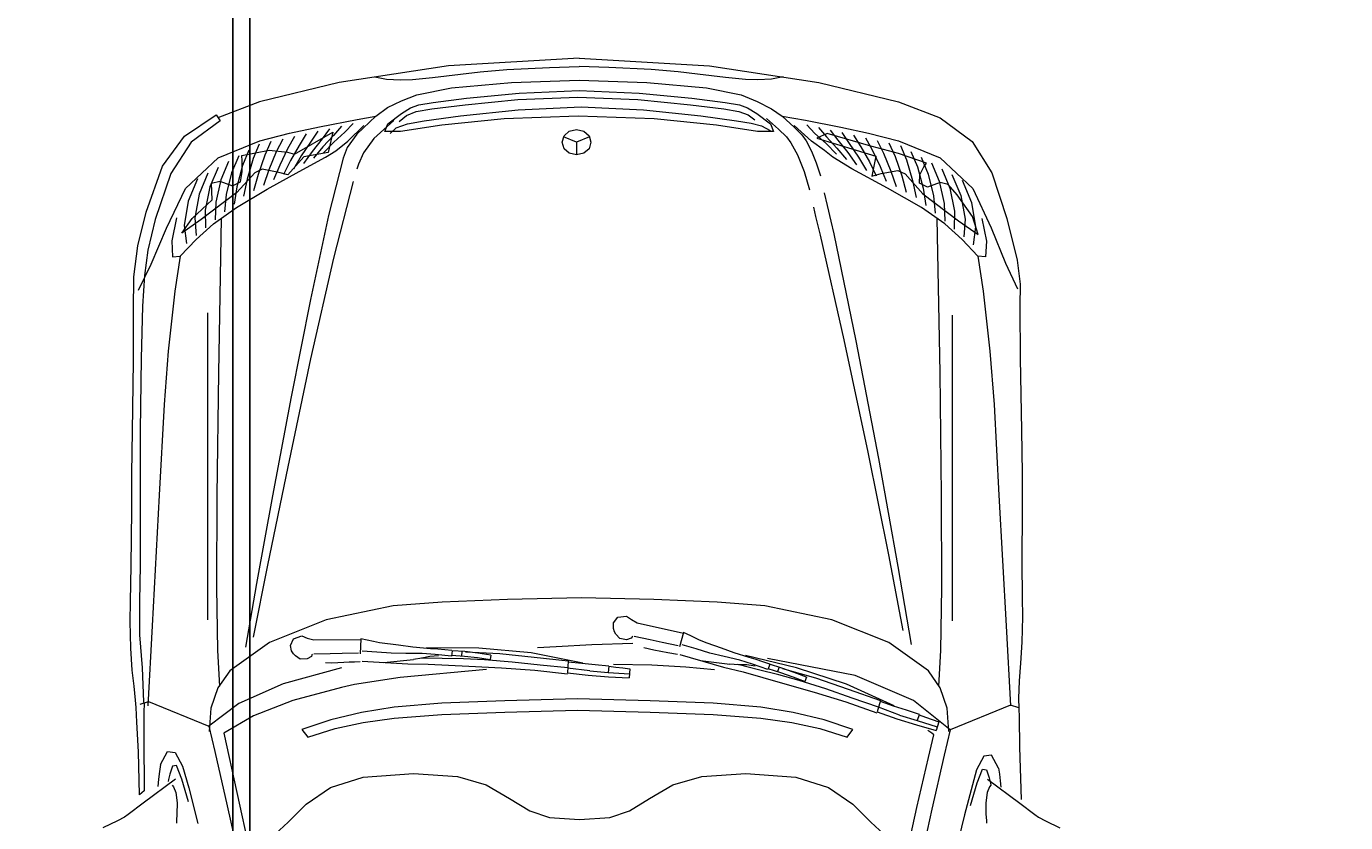
# Model space of a CAD drawing. Units: inches. Extents: x -10 to 502, y -868 to 56.
# Tile 5 of 14: x 78 to 165, y -626 to -573. Entities that reach past the tile are written whole.
import ezdxf

# ---------------------------------------------------------------- set-up
doc = ezdxf.new("R2010")
doc.units = ezdxf.units.IN
doc.header["$MEASUREMENT"] = 0
doc.layers.add('A-ANNO-DIMS', color=2, linetype='Continuous', lineweight=18)
doc.layers.add('C-PRKG-VEHI', color=8, linetype='Continuous', lineweight=13)
doc.styles.get("Standard").update_dxf_attribs({"font": 'arial.ttf'})
doc.dimstyles.get("Standard").update_dxf_attribs({"dimtxt": 0.18, "dimasz": 0.18, "dimexe": 0.18, "dimexo": 0.0625, "dimgap": 0.09, "dimtad": 0, "dimtih": 1, "dimtoh": 1, "dimdec": 0, "dimzin": 0, "dimdsep": 46, "dimlunit": 3, "dimtxsty": 'Standard', "dimcen": 0.09, "dimadec": 0, "dimazin": 0, "dimtfac": 1, "dimtdec": 0, "dimtofl": 0, "dimtmove": 0, "dimatfit": 3, "dimfxl": 1, "dimtolj": 1, "dimtzin": 0, "dimarcsym": 0})

# ---------------------------------------------------------------- blocks, each defined once
blk = doc.blocks.new('*D47')
at = {"layer": 'A-ANNO-DIMS', "color": 0, "lineweight": -2, "transparency": 16777216}
for p, q in [((91.951, -494.915), (91.951, -846.583)), ((201.951, -494.915), (201.951, -846.583)), ((92.131, -846.403), (146.622, -846.403)), ((201.771, -846.403), (147.28, -846.403))]:
    blk.add_line(p, q, dxfattribs=at)
at = {"layer": 'A-ANNO-DIMS', "color": 0, "transparency": 16777216}
for points in [[(92.131, -846.373), (92.131, -846.433), (91.951, -846.403)], [(201.771, -846.373), (201.771, -846.433), (201.951, -846.403)]]:
    blk.add_solid(points, dxfattribs=at)
at = {"layer": 'Defpoints', "color": 0, "transparency": 16777216}
for p in [(91.951, -494.853), (201.951, -494.853), (201.951, -846.403)]:
    blk.add_point(p, dxfattribs=at)
at = {"layer": 'A-ANNO-DIMS', "color": 0, "transparency": 16777216, "insert": (146.951, -846.403), "char_height": 0.18, "attachment_point": 5}
blk.add_mtext('\\A1;9\'-2"', dxfattribs=at)
blk = doc.blocks.new('*D56')
at = {"layer": 'A-ANNO-DIMS', "color": 0, "lineweight": -2, "transparency": 16777216}
for p, q in [((43.951, -549.915), (43.951, -846.583)), ((93.073, -549.915), (93.073, -846.583)), ((44.131, -846.403), (68.179, -846.403)), ((92.893, -846.403), (68.845, -846.403))]:
    blk.add_line(p, q, dxfattribs=at)
at = {"layer": 'A-ANNO-DIMS', "color": 0, "transparency": 16777216}
for points in [[(44.131, -846.373), (44.131, -846.433), (43.951, -846.403)], [(92.893, -846.373), (92.893, -846.433), (93.073, -846.403)]]:
    blk.add_solid(points, dxfattribs=at)
at = {"layer": 'Defpoints', "color": 0, "transparency": 16777216}
for p in [(43.951, -549.853), (93.073, -549.853), (43.951, -846.403)]:
    blk.add_point(p, dxfattribs=at)
at = {"layer": 'A-ANNO-DIMS', "color": 0, "transparency": 16777216, "insert": (68.512, -846.403), "char_height": 0.18, "attachment_point": 5}
blk.add_mtext('\\A1;4\'-1"', dxfattribs=at)

msp = doc.modelspace()

# ---------------------------------------------------------------- linework, layer by layer
at = {"layer": 'C-PRKG-VEHI'}
for p, q in [((106.171, -576.058), (98.969, -577.156)), ((114.77, -575.546), (106.171, -576.058)), ((110.011, -576.309), (112.816, -576.171)), ((112.816, -576.171), (114.77, -576.109)), ((114.77, -575.546), (123.37, -576.058)), ((116.725, -576.171), (114.77, -576.109)), ((119.529, -576.309), (116.725, -576.171)), ((123.37, -576.058), (130.572, -577.156)), ((101.325, -576.784), (102.091, -576.94)), ((102.091, -576.94), (102.996, -576.984)), ((102.996, -576.984), (103.8, -576.952)), ((103.8, -576.952), (105.115, -576.821)), ((105.115, -576.821), (106.967, -576.615)), ((106.967, -576.615), (108.245, -576.446)), ((108.245, -576.446), (110.011, -576.309)), ((110.311, -577.157), (114.77, -577.009)), ((114.77, -577.009), (119.229, -577.157)), ((121.296, -576.446), (119.529, -576.309)), ((122.574, -576.615), (121.296, -576.446)), ((124.426, -576.821), (122.574, -576.615)), ((125.74, -576.952), (124.426, -576.821)), ((126.545, -576.984), (125.74, -576.952)), ((127.449, -576.94), (126.545, -576.984)), ((128.216, -576.784), (127.449, -576.94)), ((98.969, -577.156), (93.718, -578.434)), ((104.081, -577.965), (106.365, -577.517)), ((106.365, -577.517), (110.311, -577.157)), ((107.344, -578.192), (110.814, -577.851)), ((110.814, -577.851), (114.77, -577.684)), ((114.77, -577.684), (118.727, -577.851)), ((118.727, -577.851), (122.196, -578.192)), ((119.229, -577.157), (123.176, -577.517)), ((123.176, -577.517), (125.459, -577.965)), ((130.572, -577.156), (135.822, -578.434)), ((93.718, -578.434), (90.973, -579.484)), ((102.159, -578.803), (103.064, -578.378)), ((103.064, -578.378), (104.081, -577.965)), ((103.665, -578.833), (104.208, -578.627)), ((104.208, -578.627), (105.15, -578.471)), ((105.064, -578.905), (107.258, -578.626)), ((105.15, -578.471), (107.344, -578.192)), ((107.258, -578.626), (110.727, -578.284)), ((110.727, -578.284), (114.684, -578.117)), ((110.76, -578.965), (114.9, -578.767)), ((114.684, -578.117), (118.641, -578.284)), ((114.9, -578.767), (119.02, -578.965)), ((118.641, -578.284), (122.11, -578.626)), ((122.11, -578.626), (124.304, -578.905)), ((122.196, -578.192), (124.391, -578.471)), ((124.391, -578.471), (125.333, -578.627)), ((125.333, -578.627), (125.876, -578.833)), ((125.459, -577.965), (126.507, -578.421)), ((126.507, -578.421), (127.442, -578.89)), ((135.822, -578.434), (138.568, -579.484)), ((88.776, -580.703), (90.853, -579.285)), ((90.853, -579.285), (91.128, -579.68)), ((97.672, -580.08), (100.158, -579.601)), ((101.381, -579.372), (100.134, -580.564)), ((100.158, -579.601), (101.381, -579.372)), ((102.557, -579.662), (101.252, -580.855)), ((101.381, -579.372), (102.159, -578.803)), ((102.166, -579.884), (103.069, -579.203)), ((102.925, -579.74), (103.394, -579.33)), ((103.069, -579.203), (103.665, -578.833)), ((103.394, -579.33), (104.035, -579.081)), ((104.035, -579.081), (105.064, -578.905)), ((104.571, -579.675), (106.949, -579.365)), ((109.825, -579.559), (105.737, -579.972)), ((106.949, -579.365), (110.76, -578.965)), ((114.714, -579.372), (109.825, -579.559)), ((119.727, -579.559), (114.714, -579.372)), ((119.02, -578.965), (122.792, -579.365)), ((123.822, -579.972), (119.727, -579.559)), ((122.792, -579.365), (125.149, -579.675)), ((124.304, -578.905), (125.301, -579.075)), ((125.301, -579.075), (125.903, -579.291)), ((125.876, -578.833), (126.472, -579.203)), ((125.903, -579.291), (126.345, -579.61)), ((126.472, -579.203), (127.374, -579.884)), ((127.12, -579.525), (127.903, -580.235)), ((127.442, -578.89), (128.16, -579.372)), ((128.16, -579.372), (128.931, -580.095)), ((128.16, -579.372), (129.695, -579.644)), ((129.695, -579.644), (132.025, -580.102)), ((138.568, -579.484), (140.669, -581.054)), ((91.128, -579.68), (89.215, -581.09)), ((93.732, -580.995), (95.699, -580.497)), ((95.699, -580.497), (97.672, -580.08)), ((96.025, -581.894), (98.543, -580.432)), ((97.567, -580.376), (97.083, -581.086)), ((98.34, -580.205), (97.838, -580.869)), ((98.543, -580.432), (98.235, -581.764)), ((99.114, -580.035), (98.593, -580.651)), ((99.348, -580.434), (98.605, -581.086)), ((99.887, -579.864), (99.348, -580.434)), ((99.536, -581.022), (100.593, -579.991)), ((101.964, -580.378), (102.166, -579.884)), ((103.012, -580.384), (101.964, -580.378)), ((102.319, -580.517), (102.711, -580.155)), ((102.711, -580.155), (103.46, -579.878)), ((105.737, -579.972), (103.012, -580.384)), ((103.46, -579.878), (104.571, -579.675)), ((113.787, -580.677), (114.127, -580.377)), ((114.127, -580.377), (114.607, -580.263)), ((114.607, -580.263), (115.086, -580.377)), ((115.086, -580.377), (115.427, -580.677)), ((126.528, -580.384), (123.822, -579.972)), ((125.149, -579.675), (126.11, -579.829)), ((126.11, -579.829), (126.787, -580.026)), ((127.576, -580.378), (126.528, -580.384)), ((126.787, -580.026), (127.358, -580.325)), ((127.374, -579.884), (127.576, -580.378)), ((127.903, -580.235), (128.433, -580.748)), ((128.931, -580.095), (129.452, -580.618)), ((130.079, -581.018), (128.948, -579.991)), ((129.767, -579.951), (130.306, -580.521)), ((130.306, -580.521), (131.049, -581.173)), ((131.111, -580.519), (130.424, -580.823)), ((130.54, -580.121), (131.061, -580.738)), ((133.985, -581.357), (131.111, -580.519)), ((131.313, -580.292), (131.816, -580.955)), ((132.025, -580.102), (133.842, -580.497)), ((132.086, -580.462), (132.571, -581.173)), ((133.842, -580.497), (135.809, -580.995)), ((87.339, -582.685), (88.776, -580.703)), ((89.215, -581.09), (87.884, -583.153)), ((90.99, -582.118), (93.732, -580.995)), ((93.702, -581.228), (93.307, -582.173)), ((94.474, -581.058), (94.062, -581.955)), ((95.248, -580.887), (94.817, -581.738)), ((96.021, -580.717), (95.572, -581.521)), ((96.327, -581.303), (95.76, -582.309)), ((96.794, -580.546), (96.327, -581.303)), ((97.083, -581.086), (96.471, -582.003)), ((97.838, -580.869), (97.182, -581.697)), ((97.894, -581.392), (97.272, -582.151)), ((98.593, -580.651), (97.894, -581.392)), ((98.605, -581.086), (97.928, -581.794)), ((98.741, -581.654), (99.536, -581.022)), ((100.134, -580.564), (99.503, -581.439)), ((101.252, -580.855), (100.559, -581.792)), ((113.657, -581.1), (113.787, -580.677)), ((113.787, -581.522), (113.657, -581.1)), ((114.607, -581.1), (113.755, -580.737)), ((115.458, -580.737), (114.607, -581.1)), ((114.607, -581.1), (114.607, -581.937)), ((115.427, -580.677), (115.556, -581.1)), ((115.556, -581.1), (115.427, -581.522)), ((128.433, -580.748), (128.723, -581.129)), ((128.723, -581.129), (129.157, -581.935)), ((129.452, -580.618), (129.735, -581.003)), ((129.735, -581.003), (130.093, -581.679)), ((130.948, -581.645), (130.079, -581.018)), ((130.424, -580.823), (134.315, -582.018)), ((131.049, -581.173), (131.725, -581.88)), ((131.061, -580.738), (131.76, -581.478)), ((131.816, -580.955), (132.471, -581.784)), ((132.571, -581.173), (133.182, -582.09)), ((132.859, -580.633), (133.326, -581.39)), ((133.326, -581.39), (133.893, -582.396)), ((133.632, -580.803), (134.081, -581.607)), ((134.488, -581.478), (133.985, -581.357)), ((134.405, -580.974), (134.836, -581.825)), ((135.179, -581.144), (135.591, -582.042)), ((135.809, -580.995), (138.551, -582.118)), ((135.952, -581.315), (136.346, -582.259)), ((140.669, -581.054), (141.962, -583.107)), ((88.835, -584.154), (90.99, -582.118)), ((92.348, -581.992), (91.881, -583.11)), ((92.56, -581.98), (94.351, -581.619)), ((92.583, -582.325), (92.56, -581.98)), ((93.025, -581.61), (92.594, -582.641)), ((93.307, -582.173), (92.915, -583.532)), ((94.062, -581.955), (93.626, -583.226)), ((94.817, -581.738), (94.338, -582.92)), ((94.351, -581.619), (95.573, -581.747)), ((95.572, -581.521), (95.049, -582.615)), ((95.573, -581.747), (96.025, -581.894)), ((96.632, -582.067), (95.592, -583.255)), ((96.471, -582.003), (95.958, -582.866)), ((96.341, -583.018), (98.062, -582.072)), ((97.182, -581.697), (96.615, -582.509)), ((98.235, -581.764), (96.632, -582.067)), ((98.062, -582.072), (98.741, -581.654)), ((99.225, -582.146), (98.272, -585.933)), ((99.503, -581.439), (99.225, -582.146)), ((100.559, -581.792), (100.239, -582.534)), ((114.127, -581.823), (113.787, -581.522)), ((114.607, -581.937), (114.127, -581.823)), ((115.086, -581.823), (114.607, -581.937)), ((115.427, -581.522), (115.086, -581.823)), ((129.157, -581.935), (129.6, -583.019)), ((130.093, -581.679), (130.4, -582.452)), ((131.479, -582.072), (130.948, -581.645)), ((132.746, -582.858), (131.479, -582.072)), ((131.76, -581.478), (132.382, -582.238)), ((132.471, -581.784), (133.038, -582.595)), ((133.182, -582.09), (133.695, -582.953)), ((134.315, -582.018), (134.061, -583.342)), ((134.081, -581.607), (134.604, -582.701)), ((135.805, -581.847), (134.488, -581.478)), ((134.836, -581.825), (135.316, -583.007)), ((135.591, -582.042), (136.027, -583.313)), ((137.647, -582.476), (135.805, -581.847)), ((136.346, -582.259), (136.738, -583.619)), ((136.629, -581.697), (137.059, -582.728)), ((137.306, -582.078), (137.772, -583.197)), ((138.551, -582.118), (140.705, -584.154)), ((86.246, -585.697), (87.339, -582.685)), ((90.317, -583.137), (89.742, -584.516)), ((90.994, -582.756), (90.455, -584.047)), ((91.671, -582.374), (91.168, -583.579)), ((91.881, -583.11), (91.531, -584.548)), ((92.594, -582.641), (92.223, -584.04)), ((93.404, -583.103), (92.235, -584.407)), ((92.464, -583.717), (92.585, -583.055)), ((92.585, -583.055), (92.583, -582.325)), ((93.894, -582.873), (93.404, -583.103)), ((94.986, -583.081), (93.894, -582.873)), ((94.338, -582.92), (93.988, -583.939)), ((94.226, -584.198), (96.341, -583.018)), ((95.049, -582.615), (94.645, -583.581)), ((95.592, -583.255), (94.986, -583.081)), ((95.76, -582.309), (95.301, -583.224)), ((100.239, -582.534), (100.126, -582.88)), ((129.6, -583.019), (129.957, -584.224)), ((130.4, -582.452), (130.668, -583.303)), ((135.088, -584.118), (132.746, -582.858)), ((133.893, -582.396), (134.352, -583.31)), ((134.604, -582.701), (135.009, -583.668)), ((134.667, -583.168), (135.759, -582.959)), ((135.316, -583.007), (135.665, -584.025)), ((135.759, -582.959), (136.249, -583.189)), ((137.059, -582.728), (137.431, -584.127)), ((137.212, -583.248), (137.48, -582.714)), ((137.48, -582.714), (137.647, -582.476)), ((137.983, -582.46), (138.485, -583.665)), ((138.659, -582.842), (139.198, -584.134)), ((141.962, -583.107), (142.956, -586.123)), ((87.884, -583.153), (86.835, -586.192)), ((89.64, -583.519), (89.029, -584.984)), ((90.561, -583.793), (91.1, -583.656)), ((90.603, -584.893), (90.561, -583.793)), ((91.168, -583.579), (90.838, -585.057)), ((91.1, -583.656), (91.936, -583.981)), ((91.936, -583.981), (92.464, -583.717)), ((92.915, -583.532), (92.674, -584.654)), ((93.626, -583.226), (93.331, -584.296)), ((99.883, -583.683), (98.586, -588.74)), ((134.061, -583.342), (134.667, -583.168)), ((136.027, -583.313), (136.322, -584.383)), ((136.249, -583.189), (137.419, -584.494)), ((136.738, -583.619), (136.979, -584.74)), ((137.19, -583.804), (137.212, -583.248)), ((137.718, -584.068), (137.19, -583.804)), ((138.553, -583.742), (137.718, -584.068)), ((137.772, -583.197), (138.123, -584.635)), ((138.485, -583.665), (138.815, -585.143)), ((139.092, -583.88), (138.553, -583.742)), ((139.669, -584.573), (139.092, -583.88)), ((139.336, -583.224), (139.911, -584.602)), ((140.014, -583.606), (140.624, -585.071)), ((87.583, -586.764), (88.835, -584.154)), ((89.742, -584.516), (89.453, -586.073)), ((92.235, -584.407), (89.881, -586.195)), ((90.455, -584.047), (90.146, -585.565)), ((91.531, -584.548), (91.42, -585.694)), ((92.223, -584.04), (92.047, -585.174)), ((92.211, -585.391), (94.226, -584.198)), ((130.91, -584.441), (131.105, -585.276)), ((137.33, -585.391), (135.088, -584.118)), ((137.419, -584.494), (139.772, -586.282)), ((137.431, -584.127), (137.606, -585.26)), ((138.123, -584.635), (138.233, -585.78)), ((139.198, -584.134), (139.508, -585.651)), ((140.682, -585.999), (139.669, -584.573)), ((139.911, -584.602), (140.2, -586.16)), ((140.705, -584.154), (141.92, -586.739)), ((85.712, -587.928), (86.246, -585.697)), ((89.029, -584.984), (88.761, -586.581)), ((89.28, -586.116), (90.603, -584.893)), ((90.146, -585.565), (90.167, -586.735)), ((90.686, -586.473), (92.211, -585.391)), ((90.838, -585.057), (90.794, -586.214)), ((130.209, -585.367), (130.354, -585.986)), ((131.105, -585.276), (131.352, -586.299)), ((138.855, -586.473), (137.33, -585.391)), ((138.815, -585.143), (138.86, -586.301)), ((139.508, -585.651), (139.487, -586.821)), ((140.624, -585.071), (140.892, -586.668)), ((86.835, -586.192), (86.356, -588.21)), ((88.249, -586.08), (87.944, -587.593)), ((88.596, -587.095), (89.28, -586.116)), ((89.881, -586.195), (88.596, -587.095)), ((88.761, -586.581), (88.913, -587.775)), ((89.453, -586.073), (89.54, -587.255)), ((89.536, -587.517), (90.686, -586.473)), ((91.198, -586.123), (91.008, -596.307)), ((98.272, -585.933), (97.085, -591.456)), ((130.354, -585.986), (130.498, -586.609)), ((130.498, -586.609), (130.643, -587.229)), ((131.352, -586.299), (131.548, -587.136)), ((138.343, -586.123), (138.533, -596.307)), ((140.005, -587.517), (138.855, -586.473)), ((139.772, -586.282), (141.057, -587.182)), ((140.2, -586.16), (140.114, -587.342)), ((141.057, -587.182), (140.682, -585.999)), ((141.307, -586.133), (141.6, -587.625)), ((142.956, -586.123), (143.637, -588.863)), ((86.581, -589.138), (87.583, -586.764)), ((130.643, -587.229), (132.212, -594.118)), ((131.548, -587.136), (133.011, -594.196)), ((140.892, -586.668), (140.741, -587.862)), ((141.92, -586.739), (142.852, -589.066)), ((85.45, -589.962), (85.712, -587.928)), ((86.356, -588.21), (86.136, -589.892)), ((87.944, -587.593), (87.991, -588.646)), ((88.498, -588.598), (89.536, -587.517)), ((141.043, -588.598), (140.005, -587.517)), ((141.6, -587.625), (141.546, -588.653)), ((85.741, -590.848), (86.581, -589.138)), ((87.991, -588.646), (88.498, -588.598)), ((88.498, -588.598), (88.146, -590.923)), ((98.586, -588.74), (97.086, -595.376)), ((141.043, -588.598), (141.395, -590.923)), ((141.546, -588.653), (141.043, -588.598)), ((142.852, -589.066), (143.654, -590.751)), ((143.637, -588.863), (143.831, -590.453)), ((85.423, -592.195), (85.45, -589.962)), ((86.136, -589.892), (86.001, -591.909)), ((88.146, -590.923), (87.706, -594.861)), ((141.395, -590.923), (141.835, -594.861)), ((143.831, -590.453), (143.8, -591.917)), ((97.085, -591.456), (95.803, -597.889)), ((85.42, -595.557), (85.423, -592.195)), ((86.001, -591.909), (85.914, -595.344)), ((90.311, -612.578), (90.311, -592.352)), ((139.373, -612.639), (139.373, -592.494)), ((143.8, -591.917), (143.818, -595.351)), ((132.212, -594.118), (133.791, -601.529)), ((133.011, -594.196), (134.492, -601.953)), ((87.706, -594.861), (87.429, -598.387)), ((141.835, -594.861), (142.112, -598.387)), ((85.354, -600.145), (85.42, -595.557)), ((85.914, -595.344), (85.866, -600.07)), ((97.086, -595.376), (95.578, -602.487)), ((143.818, -595.351), (143.912, -600.073)), ((91.008, -596.307), (90.908, -604.379)), ((138.533, -596.307), (138.633, -604.379)), ((95.803, -597.889), (94.568, -604.406)), ((87.429, -598.387), (87.114, -604.361)), ((142.112, -598.387), (142.426, -604.361)), ((85.312, -602.944), (85.354, -600.145)), ((85.866, -600.07), (85.852, -602.944)), ((143.912, -600.073), (143.968, -602.944)), ((133.791, -601.529), (135.162, -608.306)), ((134.492, -601.953), (135.777, -609.071)), ((85.301, -605.344), (85.312, -602.944)), ((85.852, -602.944), (85.854, -605.334)), ((95.578, -602.487), (94.254, -608.972)), ((143.968, -602.944), (143.956, -605.271)), ((87.114, -604.361), (86.637, -612.985)), ((90.908, -604.379), (90.89, -610.442)), ((94.568, -604.406), (93.52, -610.182)), ((138.633, -604.379), (138.65, -610.442)), ((142.426, -604.361), (142.904, -612.985)), ((85.27, -609.02), (85.301, -605.344)), ((85.854, -605.334), (85.848, -608.99)), ((143.956, -605.271), (143.943, -608.811)), ((135.162, -608.306), (136.109, -613.292)), ((85.222, -611.383), (85.27, -609.02)), ((85.848, -608.99), (85.813, -611.343)), ((94.254, -608.972), (93.308, -613.726)), ((135.777, -609.071), (136.652, -614.218)), ((143.943, -608.811), (143.968, -611.101)), ((90.89, -610.442), (90.952, -614.599)), ((93.52, -610.182), (92.802, -614.391)), ((138.65, -610.442), (138.589, -614.599)), ((85.201, -612.703), (85.222, -611.383)), ((85.813, -611.343), (85.817, -613.577)), ((102.534, -611.664), (98.11, -612.585)), ((105.759, -611.415), (102.534, -611.664)), ((110.063, -611.251), (105.759, -611.415)), ((114.925, -611.126), (110.063, -611.251)), ((119.706, -611.251), (114.925, -611.126)), ((123.862, -611.415), (119.706, -611.251)), ((127.007, -611.664), (123.862, -611.415)), ((131.431, -612.585), (127.007, -611.664)), ((143.968, -611.101), (143.989, -612.374)), ((98.11, -612.585), (94.366, -614.081)), ((117.039, -612.782), (117.329, -612.404)), ((117.329, -612.404), (117.899, -612.343)), ((117.899, -612.343), (118.218, -612.566)), ((118.218, -612.566), (118.607, -612.772)), ((135.174, -614.081), (131.431, -612.585)), ((143.989, -612.374), (143.948, -614.048)), ((85.244, -614.457), (85.201, -612.703)), ((86.637, -612.985), (86.36, -618.246)), ((117.031, -613.146), (117.039, -612.782)), ((117.102, -613.379), (117.031, -613.146)), ((117.192, -613.533), (117.102, -613.379)), ((117.459, -613.803), (117.192, -613.533)), ((118.607, -612.772), (121.64, -613.456)), ((121.656, -613.408), (121.38, -614.354)), ((122.134, -613.628), (121.656, -613.408)), ((142.904, -612.985), (143.181, -618.246)), ((85.817, -613.577), (85.981, -615.755)), ((94.366, -614.081), (91.761, -615.94)), ((95.762, -614.267), (95.96, -613.834)), ((95.836, -614.623), (95.762, -614.267)), ((95.96, -613.834), (96.501, -613.647)), ((96.501, -613.647), (96.862, -613.792)), ((96.862, -613.792), (97.288, -613.905)), ((97.288, -613.905), (100.397, -613.889)), ((100.401, -613.839), (100.345, -614.822)), ((100.803, -613.917), (100.401, -613.839)), ((101.222, -614.018), (100.803, -613.917)), ((101.625, -614.094), (101.222, -614.018)), ((102.876, -614.262), (101.625, -614.094)), ((103.82, -614.388), (102.876, -614.262)), ((104.989, -614.487), (103.82, -614.388)), ((108.176, -614.448), (104.714, -614.421)), ((113.262, -614.356), (112.022, -614.419)), ((115.601, -614.225), (113.262, -614.356)), ((118.313, -614.144), (115.601, -614.225)), ((117.903, -613.899), (117.459, -613.803)), ((118.212, -613.799), (117.903, -613.899)), ((118.259, -613.703), (118.212, -613.799)), ((118.315, -613.66), (118.259, -613.703)), ((119.455, -613.9), (118.401, -613.682)), ((119.026, -614.406), (119.693, -614.561)), ((120.24, -614.069), (119.455, -613.9)), ((121.291, -614.295), (120.24, -614.069)), ((122.483, -614.504), (121.553, -614.224)), ((122.714, -613.914), (122.134, -613.628)), ((123.199, -614.116), (122.714, -613.914)), ((124.163, -614.441), (123.199, -614.116)), ((137.78, -615.94), (135.174, -614.081)), ((143.948, -614.048), (143.856, -615.433)), ((85.337, -615.891), (85.244, -614.457)), ((90.952, -614.599), (91.086, -616.952)), ((95.958, -614.835), (95.836, -614.623)), ((96.08, -614.965), (95.958, -614.835)), ((96.401, -615.167), (96.08, -614.965)), ((96.855, -615.161), (96.401, -615.167)), ((97.134, -614.994), (96.855, -615.161)), ((97.158, -614.891), (97.134, -614.994)), ((97.203, -614.836), (97.158, -614.891)), ((98.367, -614.814), (97.292, -614.838)), ((99.171, -614.801), (98.367, -614.814)), ((100.246, -614.785), (99.171, -614.801)), ((101.454, -614.72), (100.485, -614.657)), ((102.389, -614.784), (101.454, -614.72)), ((101.914, -615.392), (103.855, -615.204)), ((103.361, -614.793), (102.389, -614.784)), ((104.425, -614.792), (103.361, -614.793)), ((104.402, -615.103), (103.855, -615.204)), ((105.757, -615.141), (104.367, -615.102)), ((104.95, -614.992), (104.402, -615.103)), ((105.289, -614.863), (104.425, -614.792)), ((105.504, -614.954), (104.95, -614.992)), ((105.456, -614.523), (104.989, -614.487)), ((106.372, -614.981), (105.289, -614.863)), ((105.932, -614.565), (105.456, -614.523)), ((107.148, -615.159), (105.757, -615.141)), ((106.398, -614.601), (105.932, -614.565)), ((106.357, -614.919), (107.212, -614.976)), ((106.405, -614.632), (106.372, -614.981)), ((107.243, -614.674), (106.386, -614.62)), ((107.046, -614.662), (107.018, -614.962)), ((108.538, -615.212), (107.148, -615.159)), ((107.212, -614.976), (108.073, -615.073)), ((108.104, -614.781), (107.243, -614.674)), ((107.299, -614.702), (109.551, -614.805)), ((108.073, -615.073), (108.923, -615.189)), ((108.955, -614.905), (108.104, -614.781)), ((111.622, -614.752), (108.176, -614.448)), ((110.37, -615.368), (108.538, -615.212)), ((108.955, -614.905), (108.907, -615.192)), ((109.551, -614.805), (111.807, -615.044)), ((115.013, -615.441), (111.622, -614.752)), ((111.807, -615.044), (114.051, -615.289)), ((114.051, -615.289), (114.006, -616.08)), ((119.693, -614.561), (120.608, -614.735)), ((120.608, -614.735), (121.259, -614.85)), ((121.402, -614.866), (124.285, -615.705)), ((123.38, -614.776), (122.483, -614.504)), ((122.78, -615.262), (124.713, -615.515)), ((124.326, -615.003), (123.38, -614.776)), ((124.996, -614.76), (124.163, -614.441)), ((125.362, -615.242), (124.326, -615.003)), ((125.98, -615.072), (124.996, -614.76)), ((126.188, -615.505), (125.362, -615.242)), ((129.094, -615.75), (125.727, -614.945)), ((126.429, -615.206), (125.98, -615.072)), ((126.882, -615.357), (126.429, -615.206)), ((132.963, -616.251), (127.18, -615.13)), ((138.589, -614.599), (138.455, -616.952)), ((85.453, -616.949), (85.337, -615.891)), ((85.981, -615.755), (86.078, -617.984)), ((91.761, -615.94), (90.976, -617.06)), ((99.113, -615.749), (95.274, -616.808)), ((98.064, -615.403), (98.464, -615.411)), ((98.464, -615.411), (98.873, -615.39)), ((98.873, -615.39), (99.275, -615.367)), ((99.275, -615.367), (99.63, -615.357)), ((99.63, -615.357), (99.985, -615.348)), ((99.985, -615.348), (100.34, -615.333)), ((100.482, -615.316), (103.48, -615.486)), ((108.667, -615.855), (102.985, -616.375)), ((103.48, -615.486), (104.819, -615.498)), ((104.819, -615.498), (106.163, -615.567)), ((106.163, -615.567), (107.501, -615.647)), ((107.501, -615.647), (109.662, -615.757)), ((109.662, -615.757), (111.855, -615.903)), ((112.199, -615.564), (110.37, -615.368)), ((111.855, -615.903), (114.005, -616.145)), ((114.028, -615.749), (112.199, -615.564)), ((114.006, -616.08), (115.364, -616.227)), ((115.488, -615.949), (114.016, -615.768)), ((114.05, -615.354), (114.942, -615.445)), ((114.942, -615.445), (115.836, -615.523)), ((115.488, -615.949), (116.697, -616.044)), ((115.836, -615.523), (116.728, -615.614)), ((116.735, -615.645), (116.697, -616.044)), ((116.697, -616.044), (118.086, -616.146)), ((116.735, -615.645), (117.193, -615.693)), ((119.573, -615.568), (117.041, -615.523)), ((117.193, -615.693), (117.652, -615.751)), ((117.652, -615.751), (118.107, -615.816)), ((118.107, -615.816), (118.081, -616.407)), ((121.799, -615.698), (119.573, -615.568)), ((123.687, -615.88), (121.799, -615.698)), ((124.285, -615.705), (125.587, -616.018)), ((125.27, -615.539), (124.713, -615.515)), ((126.581, -615.882), (125.236, -615.531)), ((125.828, -615.554), (125.27, -615.539)), ((125.587, -616.018), (126.881, -616.388)), ((126.376, -615.642), (125.828, -615.554)), ((127.216, -615.864), (126.188, -615.505)), ((127.932, -616.212), (126.581, -615.882)), ((127.327, -615.499), (126.882, -615.357)), ((127.327, -615.531), (127.216, -615.864)), ((127.216, -615.8), (128.036, -616.048)), ((128.135, -615.761), (127.311, -615.515)), ((127.945, -615.705), (127.85, -615.99)), ((128.036, -616.048), (128.853, -616.336)), ((128.95, -616.059), (128.135, -615.761)), ((128.182, -615.8), (130.353, -616.408)), ((129.751, -616.371), (128.95, -616.059)), ((132.383, -616.822), (129.094, -615.75)), ((138.565, -617.06), (137.78, -615.94)), ((143.856, -615.433), (143.764, -616.606)), ((85.552, -617.871), (85.453, -616.949)), ((95.274, -616.808), (92.36, -618.109)), ((99.987, -616.844), (99.113, -617.048)), ((102.985, -616.375), (99.987, -616.844)), ((115.364, -616.227), (116.718, -616.333)), ((116.718, -616.333), (118.081, -616.407)), ((126.881, -616.388), (128.166, -616.767)), ((129.275, -616.577), (127.932, -616.212)), ((128.166, -616.767), (130.247, -617.361)), ((128.853, -616.336), (129.656, -616.64)), ((131.025, -617.14), (129.275, -616.577)), ((129.751, -616.371), (129.64, -616.64)), ((130.353, -616.408), (132.497, -617.148)), ((135.533, -618.256), (132.383, -616.822)), ((136.796, -617.911), (132.963, -616.251)), ((143.764, -616.606), (143.722, -617.767)), ((85.6, -618.365), (85.552, -617.871)), ((90.976, -617.06), (90.515, -618.416)), ((95.913, -617.892), (93.327, -618.903)), ((99.113, -617.048), (95.913, -617.892)), ((114.665, -617.798), (109.883, -617.923)), ((119.446, -617.923), (114.665, -617.798)), ((130.247, -617.361), (132.352, -617.996)), ((132.762, -617.743), (131.025, -617.14)), ((132.497, -617.148), (134.63, -617.891)), ((134.503, -618.335), (132.762, -617.743)), ((134.63, -617.891), (134.408, -618.652)), ((139.026, -618.416), (138.565, -617.06)), ((143.722, -617.767), (143.743, -618.415)), ((85.648, -619.331), (85.6, -618.365)), ((85.856, -618.144), (86.415, -617.976)), ((86.078, -617.984), (86.098, -618.029)), ((86.103, -618.636), (86.089, -620.404)), ((86.098, -618.029), (86.11, -618.081)), ((86.116, -618.139), (86.103, -618.636)), ((86.11, -618.081), (86.116, -618.139)), ((86.415, -617.976), (90.386, -619.598)), ((92.36, -618.109), (90.386, -619.598)), ((90.515, -618.416), (90.411, -619.934)), ((100.448, -618.683), (98.41, -619.182)), ((102.583, -618.335), (100.448, -618.683)), ((105.727, -618.087), (102.583, -618.335)), ((109.883, -617.923), (105.727, -618.087)), ((105.727, -618.823), (109.883, -618.659)), ((109.883, -618.659), (114.665, -618.534)), ((114.665, -618.534), (119.446, -618.659)), ((123.602, -618.087), (119.446, -617.923)), ((119.446, -618.659), (123.602, -618.823)), ((126.747, -618.335), (123.602, -618.087)), ((128.881, -618.683), (126.747, -618.335)), ((130.919, -619.182), (128.881, -618.683)), ((132.352, -617.996), (134.392, -618.715)), ((134.408, -618.652), (135.698, -619.1)), ((135.881, -618.858), (134.487, -618.351)), ((134.614, -617.955), (135.463, -618.244)), ((135.463, -618.244), (136.315, -618.521)), ((136.315, -618.521), (137.164, -618.81)), ((139.212, -619.837), (136.796, -617.911)), ((139.13, -619.934), (139.026, -618.416)), ((143.182, -618.215), (139.212, -619.837)), ((143.741, -618.383), (143.182, -618.215)), ((143.743, -618.415), (143.752, -619.025)), ((85.739, -621.276), (85.648, -619.331)), ((90.386, -619.598), (90.769, -621.259)), ((93.327, -618.903), (91.361, -620.053)), ((98.41, -619.182), (96.517, -619.812)), ((98.697, -619.743), (100.548, -619.358)), ((100.548, -619.358), (102.583, -619.072)), ((102.583, -619.072), (105.727, -618.823)), ((123.602, -618.823), (126.747, -619.072)), ((126.747, -619.072), (128.781, -619.358)), ((128.781, -619.358), (130.633, -619.743)), ((132.813, -619.812), (130.919, -619.182)), ((135.698, -619.1), (136.993, -619.509)), ((135.881, -618.858), (137.038, -619.222)), ((136.993, -619.509), (138.305, -619.887)), ((137.164, -618.842), (137.038, -619.222)), ((137.038, -619.222), (138.368, -619.634)), ((137.164, -618.842), (137.6, -618.992)), ((137.6, -618.992), (138.034, -619.151)), ((138.034, -619.151), (138.463, -619.317)), ((138.463, -619.317), (138.305, -619.887)), ((143.752, -619.025), (143.795, -620.974)), ((86.089, -620.404), (86.116, -623.863)), ((91.361, -620.053), (94.882, -636.132)), ((96.517, -619.812), (96.903, -620.31)), ((96.903, -620.31), (98.697, -619.743)), ((130.633, -619.743), (132.427, -620.31)), ((132.427, -620.31), (132.813, -619.812)), ((137.885, -619.958), (137.75, -619.871)), ((137.792, -621.667), (138.146, -620.156)), ((138.017, -620.054), (137.885, -619.958)), ((138.146, -620.156), (138.017, -620.054)), ((139.212, -619.837), (138.828, -621.498)), ((85.813, -624.123), (85.739, -621.276)), ((87.198, -622.114), (87.649, -621.261)), ((87.649, -621.261), (88.163, -621.327)), ((88.163, -621.327), (88.652, -622.226)), ((90.769, -621.259), (91.587, -624.834)), ((143.795, -620.974), (143.902, -624.435)), ((87.198, -622.114), (87.13, -622.592)), ((87.981, -622.226), (87.809, -622.761)), ((88.244, -622.189), (87.981, -622.226)), ((88.594, -623.084), (88.244, -622.189)), ((88.652, -622.226), (89.054, -623.65)), ((137.028, -624.963), (137.792, -621.667)), ((138.828, -621.498), (138.01, -625.073)), ((141.434, -621.567), (140.945, -622.466)), ((141.947, -621.5), (141.434, -621.567)), ((142.399, -622.354), (141.947, -621.5)), ((88.184, -623.081), (86.047, -624.678)), ((87.071, -623.078), (87.02, -623.574)), ((87.13, -622.592), (87.071, -623.078)), ((87.724, -623.109), (87.701, -623.233)), ((87.809, -622.761), (87.724, -623.109)), ((89.043, -624.575), (88.594, -623.084)), ((98.397, -623.63), (100.551, -622.948)), ((100.551, -622.948), (103.858, -622.716)), ((103.858, -622.716), (106.758, -622.911)), ((106.758, -622.911), (108.648, -623.47)), ((120.958, -623.47), (122.848, -622.911)), ((122.848, -622.911), (125.748, -622.716)), ((125.748, -622.716), (129.056, -622.948)), ((129.056, -622.948), (131.209, -623.63)), ((140.945, -622.466), (140.152, -625.432)), ((141.003, -623.323), (141.353, -622.428)), ((141.353, -622.428), (141.616, -622.466)), ((141.616, -622.466), (141.788, -623)), ((141.672, -623.081), (143.809, -624.678)), ((141.788, -623), (141.873, -623.348)), ((142.399, -622.354), (142.458, -622.768)), ((142.458, -622.768), (142.511, -623.189)), ((86.116, -623.863), (85.813, -624.123)), ((87.961, -623.472), (88.048, -623.59)), ((88.048, -623.59), (88.209, -623.969)), ((88.209, -623.969), (88.296, -624.647)), ((89.054, -623.65), (89.645, -626.004)), ((96.796, -624.744), (98.397, -623.63)), ((108.648, -623.47), (110.186, -624.356)), ((119.42, -624.356), (120.958, -623.47)), ((131.209, -623.63), (132.81, -624.744)), ((140.554, -624.814), (141.003, -623.323)), ((141.647, -623.969), (141.56, -624.647)), ((141.809, -623.59), (141.647, -623.969)), ((141.896, -623.472), (141.809, -623.59)), ((141.873, -623.348), (141.896, -623.472)), ((142.511, -623.189), (142.558, -623.617)), ((86.047, -624.678), (85.065, -625.417)), ((88.296, -624.647), (88.282, -625.367)), ((91.587, -624.834), (92.343, -628.21)), ((95.608, -625.916), (96.796, -624.744)), ((110.186, -624.356), (111.518, -625.174)), ((118.089, -625.174), (119.42, -624.356)), ((132.81, -624.744), (133.998, -625.916)), ((141.56, -624.647), (141.575, -625.367)), ((143.809, -624.678), (144.791, -625.417)), ((84.829, -625.597), (84.355, -625.827)), ((85.065, -625.417), (84.829, -625.597)), ((88.282, -625.367), (88.255, -625.827)), ((111.518, -625.174), (112.82, -625.609)), ((112.82, -625.609), (114.803, -625.736)), ((114.803, -625.736), (116.786, -625.609)), ((116.786, -625.609), (118.089, -625.174)), ((136.301, -628.19), (137.028, -624.963)), ((138.01, -625.073), (137.254, -628.449)), ((140.152, -625.432), (139.073, -629.901)), ((141.575, -625.367), (141.602, -625.827)), ((144.791, -625.417), (145.027, -625.597)), ((145.027, -625.597), (145.502, -625.826)), ((84.355, -625.827), (83.408, -626.292)), ((88.255, -625.827), (88.24, -625.989)), ((94.753, -626.702), (95.608, -625.916)), ((133.998, -625.916), (134.853, -626.702)), ((141.602, -625.827), (141.616, -625.989)), ((145.502, -625.826), (146.449, -626.291))]:
    msp.add_line(p, q, dxfattribs=at)

# ---------------------------------------------------------------- dimensions: what is measured, and where the dimension line sits
at = {"layer": 'A-ANNO-DIMS'}
for base, p1, p2, picture, middle in [((201.951, -846.403), (91.951, -494.853), (201.951, -494.853), '*D47', (146.951, -846.403)), ((43.951, -846.403), (93.073, -549.853), (43.951, -549.853), '*D56', (68.512, -846.403))]:
    dim = msp.add_linear_dim(base=base, p1=p1, p2=p2, dimstyle='Standard', override={"dimdec": 1, "dimlfac": 1, "dimrnd": 0, "dimzin": 1, "dimdsep": 46, "dimlunit": 4, "dimfrac": 2}, dxfattribs=at)
    dim.commit()
    dim.dimension.update_dxf_attribs({"geometry": picture, "text_midpoint": middle})

doc.saveas('drawing.dxf')
